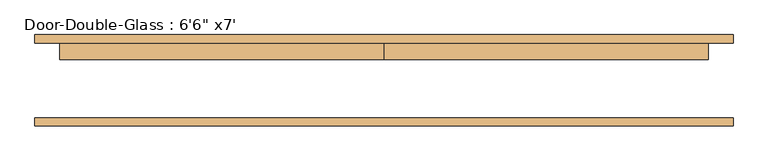
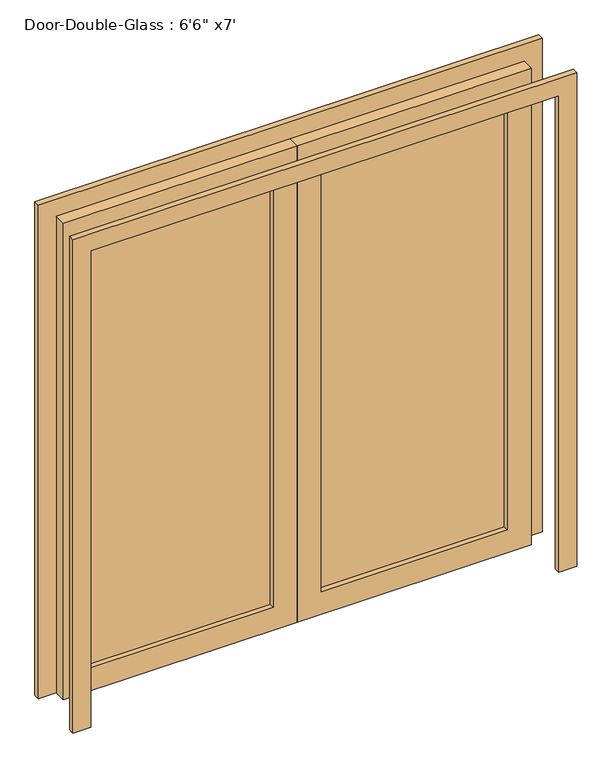
"""IFC4 building model written with IfcOpenShell, lengths in millimetres: door geometry."""

from ifc_helpers import new_model, si_unit, frame, origin, place, context, project, spatial, polyline, outline, extrude, source, transform, mapped, element, save


def door_f6d125f6(model_context):
    return source(origin(), model_context, "Body", "SweptSolid", [
        extrude(outline(polyline([(2133.6, 990.6), (2133.6, 0.0), (0.0, 0.0), (0.0, 990.6), (2133.6, 990.6)]), holes=[polyline([(2032.0, 889.0), (101.6, 889.0), (101.6, 101.6), (2032.0, 101.6), (2032.0, 889.0)])]), frame((0.0, 65.88125, 0.0), z_axis=(0.0, 1.0, 0.0), x_axis=(0.0, 0.0, 1.0)), (0.0, 0.0, 1.0), 50.8),
        extrude(outline(polyline([(2133.6, -990.6), (0.0, -990.6), (0.0, 0.0), (2133.6, 0.0), (2133.6, -990.6)]), holes=[polyline([(2032.0, -889.0), (2032.0, -101.6), (101.6, -101.6), (101.6, -889.0), (2032.0, -889.0)])]), frame((0.0, 65.88125, 0.0), z_axis=(0.0, 1.0, 0.0), x_axis=(0.0, 0.0, 1.0)), (0.0, 0.0, 1.0), 50.8),
        extrude(outline(polyline([(-889.0, 94.45625), (-101.6, 94.45625), (-101.6, 88.10625), (-889.0, 88.10625), (-889.0, 94.45625)])), frame((0.0, 0.0, 101.6), z_axis=(0.0, 0.0, 1.0), x_axis=(1.0, 0.0, 0.0)), (0.0, 0.0, 1.0), 1930.4),
        extrude(outline(polyline([(101.6, 94.45625), (889.0, 94.45625), (889.0, 88.10625), (101.6, 88.10625), (101.6, 94.45625)])), frame((0.0, 0.0, 101.6), z_axis=(0.0, 0.0, 1.0), x_axis=(1.0, 0.0, 0.0)), (0.0, 0.0, 1.0), 1930.4),
        extrude(outline(polyline([(0.0, 1066.8), (2209.8, 1066.8), (2209.8, -1066.8), (0.0, -1066.8), (0.0, -990.6), (2133.6, -990.6), (2133.6, 990.6), (0.0, 990.6), (0.0, 1066.8)])), frame((0.0, -137.31875, 0.0), z_axis=(0.0, 1.0, 0.0), x_axis=(0.0, 0.0, 1.0)), (0.0, 0.0, 1.0), 25.4),
        extrude(outline(polyline([(0.0, 1066.8), (2209.8, 1066.8), (2209.8, -1066.8), (0.0, -1066.8), (0.0, -990.6), (2133.6, -990.6), (2133.6, 990.6), (0.0, 990.6), (0.0, 1066.8)])), frame((0.0, 116.68125, 0.0), z_axis=(0.0, 1.0, 0.0), x_axis=(0.0, 0.0, 1.0)), (0.0, 0.0, 1.0), 25.4),
    ])


if __name__ == "__main__":
    model = new_model("IFC4")
    model_context = context("Model", 3, world=origin())
    ifc_project = project(units=[si_unit("LENGTHUNIT", "METRE", prefix="MILLI")], contexts=[model_context])
    site = spatial("IfcSite", under=ifc_project)
    building = spatial("IfcBuilding", under=site)
    placement = place(None, origin())
    door_shape = door_f6d125f6(model_context)
    element("IfcDoor", 1, ObjectType="Door-Double-Glass : 6'6\" x7'", at=placement, inside=building, context=model_context, shape_type="MappedRepresentation", body=[
        mapped(door_shape, transform((0.0, 0.0, 0.0), x_axis=(1.0, 0.0, 0.0), y_axis=(0.0, 1.0, 0.0), z_axis=(0.0, 0.0, 1.0))),
    ])
    save(model, "model.ifc")

# Revit data of these elements
# Type "Door-Double-Glass : 6'6\" x7'"
#   Type Mark = "29"
#   Construction Type Id = "opn-d45"
#   Assembly Code = "C1020"
#   Analytic Construction = "Wood frame, double glass door "
#   W = 3' - 3"
#   Thickness = 0' - 2"
#   Thermal Resistance (R) = 1.8150 (h·ft²·°F)/BTU
#   Swing Angle [instance default] = 90.00°
#   Heat Transfer Coefficient (U) = 0.5510 BTU/(h·ft²·°F)
#   Height = 7' - 0"
#   Bottom Rail = 0' - 4"
#   Top Rail = 0' - 4"
#   Stiles = 0' - 4"
#   Trim Projection = 0' - 1"
#   Trim Width = 0' - 3"
#   Width = 6' - 6"
#   Define Thermal Properties by = 1
#   Glazing = Glass
#   Panel Material = Wood - Birch - Solid Stained Light Low Gloss
#   Trim Material = Paint - Sienna
#   Visual Light Transmittance = 0
#   Solar Heat Gain Coefficient = 0
#   Function = (empty or 0)
#   Wall Closure = (empty or 0)
# Element 1 (IfcDoor, "Door-Double-Glass : 6'6\" x7'")
#   Materials on its faces: "Wood - Birch - Solid Stained Light Low Gloss", "Paint - Sienna", "Glass"
# Materials
#   "Glass": class "Glass", colour RGB 0 128 192, transparency 0.75, Description = "Soda Lime Glass", Cost = 0
#   "Wood - Birch - Solid Stained Light Low Gloss": class "Wood", colour RGB 210 159 95, transparency 0, Cost = 0
#   "Paint - Sienna": colour RGB 118 70 51, transparency 0, Cost = 0
